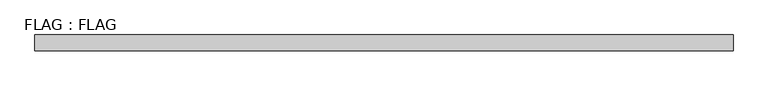
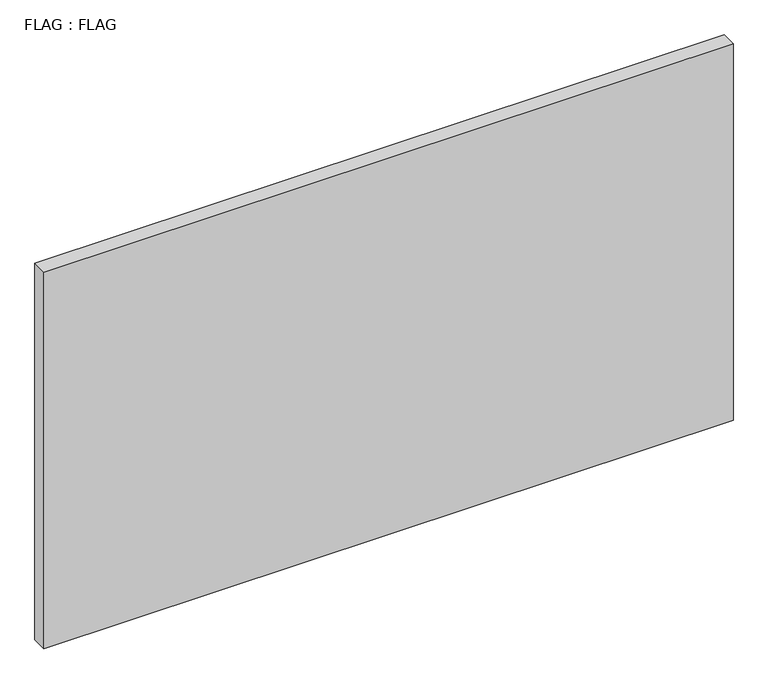
"""IFC4 building model written with IfcOpenShell, lengths in millimetres: proxy geometry, FLAG : FLAG."""

from ifc_helpers import new_model, si_unit, frame, origin, place, context, project, spatial, polyline, outline, extrude, source, transform, mapped, element, save


def flag_flag_4961f895(model_context):
    return source(origin(), model_context, "Body", "SweptSolid", [
        extrude(outline(polyline([(-33833.1287293, 994.8102334), (-33833.1287293, 944.0102334), (-36084.8798108, 944.0102334), (-36084.8798108, 994.8102334), (-33833.1287293, 994.8102334)])), frame((0.0, 0.0, 4584.3359094), z_axis=(0.0, 0.0, 1.0), x_axis=(1.0, 0.0, 0.0)), (0.0, 0.0, 1.0), 1300.5976778),
    ])


if __name__ == "__main__":
    model = new_model("IFC4")
    model_context = context("Model", 3, world=origin())
    ifc_project = project(units=[si_unit("LENGTHUNIT", "METRE", prefix="MILLI")], contexts=[model_context])
    site = spatial("IfcSite", under=ifc_project)
    building = spatial("IfcBuilding", under=site)
    placement = place(None, origin())
    flag_flag_shape = flag_flag_4961f895(model_context)
    element("IfcBuildingElementProxy", 1, Name="FLAG : FLAG", ObjectType="FLAG : FLAG", at=placement, inside=building, context=model_context, shape_type="MappedRepresentation", body=[
        mapped(flag_flag_shape, transform((0.0, 0.0, 0.0), x_axis=(1.0, 0.0, 0.0), y_axis=(0.0, 1.0, 0.0), z_axis=(0.0, 0.0, 1.0))),
    ])
    save(model, "model.ifc")
